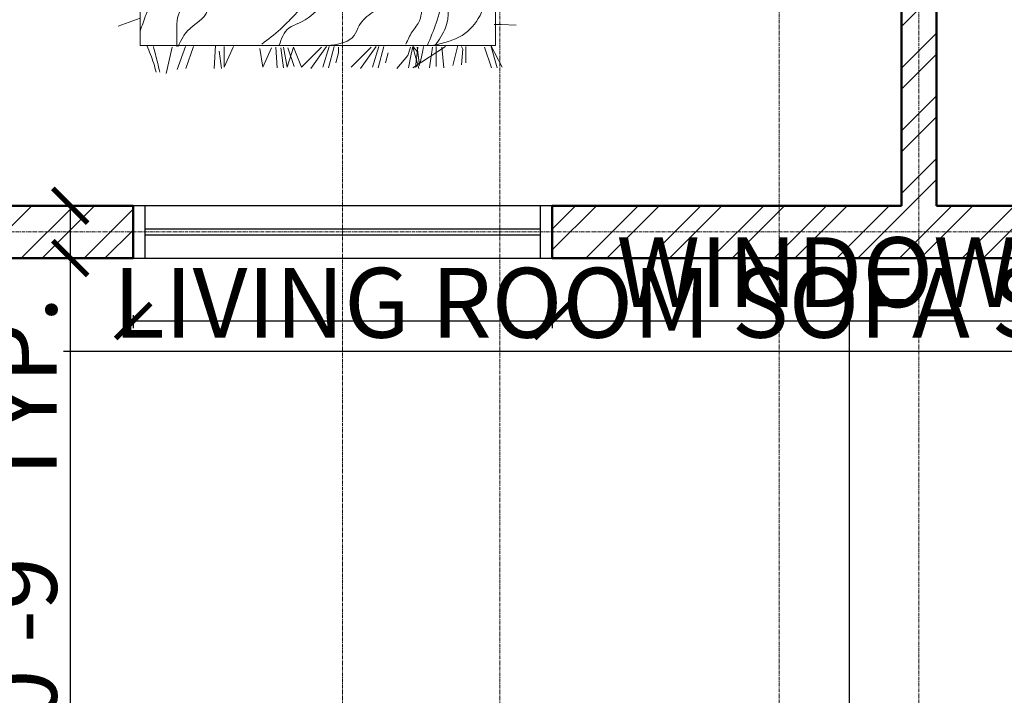
# Model space of a CAD drawing. Units: inches. Extents: x 261 to 2725, y 291 to 1454.
# Tile 4 of 35: x 519 to 688, y 433 to 549. Entities that reach past the tile are written whole.
import ezdxf

# ---------------------------------------------------------------- set-up
doc = ezdxf.new("R2010")
doc.units = ezdxf.units.IN
doc.linetypes.add('CENTER', pattern=[2, 1.25, -0.25, 0.25, -0.25])
for name, color, linetype, lineweight in [('A-ANNO-DIMS', 136, 'Continuous', 18), ('A-FLOR-STRS', 42, 'Continuous', 25), ('A-FURN', 30, 'Continuous', 18), ('A-GLAZ', 150, 'Continuous', 25), ('A-GRID', 251, 'CENTER', 13), ('A-WALL', 222, 'Continuous', 50), ('A-WALL-PATT', 243, 'Continuous', 13)]:
    doc.layers.add(name, color=color, linetype=linetype, lineweight=lineweight)
doc.styles.get("Standard").update_dxf_attribs({"font": 'arial.ttf'})
doc.dimstyles.new('ISO-25', dxfattribs={"dimtxt": 12, "dimasz": 6, "dimexe": 1.25, "dimexo": 0.625, "dimtad": 1, "dimdec": 0, "dimlunit": 3, "dimtxsty": 'Standard', "dimblk": 'ARCHTICK', "dimcen": 2.5, "dimadec": 0, "dimazin": 0, "dimtfac": 1, "dimtdec": 0, "dimtmove": 0, "dimatfit": 3, "dimfxl": 1, "dimfxlon": 1, "dimarcsym": 0})

# ---------------------------------------------------------------- blocks, each defined once
blk = doc.blocks.new('A$C2B723114')
for p, q in [((0.5047, 1.5819), (0.5353, 1.4945)), ((0.4269, 0.0884), (0.4269, 1.4945)), ((0.4269, 1.4945), (0.6794, 1.4945)), ((0.3172, 1.3923), (0.4213, 1.3687)), ((0.3318, 1.3485), (0.4241, 1.3149)), ((0.3367, 1.3143), (0.4241, 1.2838)), ((0.3367, 1.2016), (0.427, 1.1959)), ((0.3367, 1.1724), (0.405, 1.1821)), ((0.4241, 1.162), (0.3421, 1.162)), ((0.3421, 1.162), (0.4241, 1.1252)), ((0.4157, 1.0206), (0.3421, 1.0093)), ((0.3421, 1.0093), (0.4185, 0.9754)), ((0.4213, 0.9584), (0.3392, 0.9527)), ((0.4185, 0.9386), (0.3392, 0.9272)), ((0.4213, 0.9272), (0.3421, 0.9131)), ((0.3421, 0.9131), (0.4213, 0.8876)), ((0.4185, 0.9103), (0.3449, 0.8848)), ((0.4213, 0.8876), (0.3421, 0.8565)), ((0.3364, 0.8197), (0.4241, 0.7574)), ((0.3421, 0.8565), (0.4213, 0.7772)), ((0.3392, 0.7489), (0.4241, 0.7263)), ((0.3421, 0.7716), (0.4241, 0.7461)), ((0.359, 0.7206), (0.3987, 0.7093)), ((0.3987, 0.7093), (0.4213, 0.7093)), ((0.3421, 0.6601), (0.4213, 0.5808)), ((0.3364, 0.6233), (0.4241, 0.561)), ((0.3392, 0.5525), (0.4241, 0.5299)), ((0.3421, 0.5752), (0.4241, 0.5497)), ((0.359, 0.5242), (0.3987, 0.5129)), ((0.3364, 0.4785), (0.3874, 0.436)), ((0.3392, 0.4332), (0.393, 0.4219)), ((0.3874, 0.436), (0.4213, 0.4247)), ((0.4213, 0.415), (0.3364, 0.3923)), ((0.4241, 0.2868), (0.3392, 0.415)), ((0.3421, 0.4049), (0.3647, 0.3851)), ((0.4213, 0.3964), (0.3421, 0.4049)), ((0.4213, 0.398), (0.3477, 0.3895)), ((0.393, 0.4219), (0.4241, 0.4162)), ((0.4241, 0.4162), (0.4015, 0.3964)), ((0.3647, 0.3851), (0.4072, 0.3766)), ((0.4072, 0.3766), (0.4241, 0.3738)), ((0.4213, 0.3377), (0.3392, 0.3491)), ((0.4241, 0.3236), (0.3449, 0.3236)), ((0.3392, 0.2925), (0.4213, 0.3009)), ((0.3477, 0.2571), (0.427, 0.2373)), ((0.3506, 0.2231), (0.4128, 0.2175)), ((0.359, 0.2061), (0.4241, 0.2061)), ((0.4128, 0.2175), (0.4241, 0.2231)), ((0.3392, 0.1042), (0.4213, 0.1325)), ((0.3392, 0.0815), (0.427, 0.107)), ((0.427, 0.107), (0.3421, 0.0617)), ((2.4685, 0.0903), (0.4269, 0.0884)), ((0.5106, 0.094), (0.5106, 0.0657)), ((0.5106, 0.0657), (0.5077, 0.0063))]:
    blk.add_line(p, q)
for points, knots in [([(0.6768, 1.3104), (0.6615, 1.3339), (0.6315, 1.3797), (0.604, 1.4501), (0.5417, 1.4748), (0.5064, 1.4871), (0.4848, 1.4945)], [0, 0, 0, 0, 110.980521, 216.571322, 273.316778, 363.252298, 363.252298, 363.252298, 363.252298]), ([(0.427, 1.4678), (0.4036, 1.4582), (0.3693, 1.4441), (0.3335, 1.4344), (0.3221, 1.4313)], [0, 0, 0, 0, 98.452083, 144.639601, 144.639601, 144.639601, 144.639601]), ([(0.4241, 1.4423), (0.4031, 1.437), (0.3691, 1.4284), (0.3351, 1.4199), (0.3221, 1.4167)], [0, 0, 0, 0, 84.638756, 136.955563, 136.955563, 136.955563, 136.955563]), ([(0.6768, 1.286), (0.6567, 1.2911), (0.6145, 1.3017), (0.5543, 1.3533), (0.4816, 1.349), (0.4362, 1.3493), (0.4233, 1.3493)], [0, 0, 0, 0, 80.250278, 168.388677, 295.908361, 346.663112, 346.663112, 346.663112, 346.663112]), ([(0.4233, 1.3445), (0.4367, 1.3385), (0.464, 1.3264), (0.5129, 1.2848), (0.5456, 1.2161), (0.6131, 1.2349), (0.6142, 1.1913), (0.6642, 1.1806), (0.674, 1.144), (0.6817, 1.1154)], [0, 0, 0, 0, 56.745495, 115.23739, 254.956954, 286.678662, 337.828324, 366.201072, 468.500395, 468.500395, 468.500395, 468.500395]), ([(0.6817, 0.8034), (0.6673, 0.8119), (0.6341, 0.8315), (0.5785, 0.8518), (0.5349, 0.8973), (0.4828, 0.9461), (0.4518, 0.9879), (0.4331, 1.013)], [0, 0, 0, 0, 65.318952, 150.437229, 226.833166, 307.58338, 429.454095, 429.454095, 429.454095, 429.454095]), ([(0.4282, 0.9448), (0.4547, 0.9353), (0.496, 0.9206), (0.5223, 0.8436), (0.5628, 0.7946), (0.6113, 0.7575), (0.6214, 0.7173), (0.6539, 0.7022), (0.672, 0.6897), (0.6768, 0.6864)], [0, 0, 0, 0, 102.299436, 159.044876, 303.717955, 348.579152, 391.138254, 454.581655, 477.456496, 477.456496, 477.456496, 477.456496]), ([(0.4282, 0.74), (0.4347, 0.7029), (0.444, 0.6496), (0.5194, 0.6274), (0.555, 0.5807), (0.5975, 0.5243), (0.6789, 0.5415), (0.677, 0.5095), (0.6768, 0.5061)], [0, 0, 0, 0, 130.791737, 187.537266, 286.231946, 353.673191, 460.023761, 472.712403, 472.712403, 472.712403, 472.712403]), ([(0.4331, 0.4427), (0.4498, 0.4356), (0.4827, 0.4216), (0.5314, 0.3759), (0.632, 0.3884), (0.6996, 0.3513), (0.7423, 0.3278)], [0, 0, 0, 0, 70.931849, 139.556414, 248.154027, 434.709995, 434.709995, 434.709995, 434.709995]), ([(2.4625, 0.1088), (2.4095, 0.1438), (2.2904, 0.2226), (2.0623, 0.1771), (1.9006, 0.2246), (1.7699, 0.2337), (1.6941, 0.2766), (1.5528, 0.2786), (1.4005, 0.2587), (1.2324, 0.3267), (1.059, 0.2939), (0.9218, 0.426), (0.7359, 0.3204), (0.5586, 0.2391), (0.4502, 0.3116), (0.427, 0.3272)], [0, 0, 0, 0, 239.874704, 538.942419, 850.40885, 893.390315, 1047.998294, 1176.505142, 1437.500972, 1637.333004, 1864.324391, 2089.058767, 2248.736533, 2637.953392, 2744.252142, 2744.252142, 2744.252142, 2744.252142]), ([(1.9771, 0.0962), (1.9286, 0.1117), (1.7864, 0.157), (1.5223, 0.1992), (1.2611, 0.141), (1.0527, 0.2023), (0.8859, 0.1885), (0.76, 0.3042), (0.6211, 0.292), (0.5187, 0.3203), (0.4572, 0.3456), (0.4282, 0.3575)], [0, 0, 0, 0, 198.710624, 582.73994, 1031.873213, 1206.082894, 1423.278209, 1655.952104, 1808.744089, 1945.69963, 2068.229211, 2068.229211, 2068.229211, 2068.229211]), ([(0.8474, 0.0943), (0.82, 0.1047), (0.757, 0.1287), (0.6201, 0.1029), (0.4623, 0.1837), (0.4372, 0.2936), (0.4282, 0.3331)], [0, 0, 0, 0, 112.422038, 258.341957, 533.791494, 688.286079, 688.286079, 688.286079, 688.286079])]:
    blk.add_open_spline(points, degree=3, knots=knots)
blk = doc.blocks.new('_ArchTick')
at = {"color": 0, "linetype": 'ByBlock', "const_width": 0.15}
blk.add_lwpolyline([(-0.5, -0.5), (0.5, 0.5)], dxfattribs=at)
blk = doc.blocks.new('*D28')
at = {"layer": 'A-ANNO-DIMS', "color": 0, "lineweight": -2, "transparency": 16777216}
for p, q in [((469.45, 349.55), (469.45, 347.3)), ((469.45, 348.55), (955.45, 348.55)), ((955.45, 349.55), (955.45, 347.3))]:
    blk.add_line(p, q, dxfattribs=at)
at = {"layer": 'Defpoints', "color": 0, "transparency": 16777216}
for p in [(469.45, 508.47), (955.45, 508.47), (955.45, 348.55)]:
    blk.add_point(p, dxfattribs=at)
at = {"layer": 'A-ANNO-DIMS', "color": 0, "lineweight": -2, "transparency": 16777216, "xscale": 6, "yscale": 6, "zscale": 6, "rotation": 180}
blk.add_blockref('_ArchTick', (469.45, 348.55), dxfattribs=at)
at = {"layer": 'A-ANNO-DIMS', "color": 0, "lineweight": -2, "transparency": 16777216, "xscale": 6, "yscale": 6, "zscale": 6}
blk.add_blockref('_ArchTick', (955.45, 348.55), dxfattribs=at)
at = {"layer": 'A-ANNO-DIMS', "color": 0, "transparency": 16777216, "insert": (712.45, 355.3), "char_height": 12, "attachment_point": 5}
blk.add_mtext('40\'-6"', dxfattribs=at)
blk = doc.blocks.new('*D31')
at = {"layer": 'A-ANNO-DIMS', "color": 0, "lineweight": -2, "transparency": 16777216}
for p, q in [((478.45, 389.14), (478.45, 386.89)), ((946.45, 389.14), (946.45, 386.89)), ((478.45, 388.14), (946.45, 388.14))]:
    blk.add_line(p, q, dxfattribs=at)
at = {"layer": 'Defpoints', "color": 0, "transparency": 16777216}
for p in [(478.45, 517.47), (946.45, 517.47), (946.45, 388.14)]:
    blk.add_point(p, dxfattribs=at)
at = {"layer": 'A-ANNO-DIMS', "color": 0, "lineweight": -2, "transparency": 16777216, "xscale": 6, "yscale": 6, "zscale": 6, "rotation": 180}
blk.add_blockref('_ArchTick', (478.45, 388.14), dxfattribs=at)
at = {"layer": 'A-ANNO-DIMS', "color": 0, "lineweight": -2, "transparency": 16777216, "xscale": 6, "yscale": 6, "zscale": 6}
blk.add_blockref('_ArchTick', (946.45, 388.14), dxfattribs=at)
at = {"layer": 'A-ANNO-DIMS', "color": 0, "transparency": 16777216, "insert": (712.45, 394.89), "char_height": 12, "attachment_point": 5}
blk.add_mtext("39'", dxfattribs=at)
blk = doc.blocks.new('WIN-72')
for p, q in [((955.45, 950.47), (946.45, 950.47)), ((950.45, 950.47), (950.45, 882.47)), ((951.45, 882.47), (951.45, 950.47)), ((946.45, 882.47), (955.45, 882.47))]:
    blk.add_line(p, q)
blk.add_lwpolyline([(955.45, 880.47), (955.45, 952.47), (946.45, 952.47), (946.45, 880.47)], close=True)
blk = doc.blocks.new('*D39')
at = {"layer": 'A-ANNO-DIMS', "color": 0, "lineweight": -2, "ltscale": 0.07, "transparency": 16777216}
for p, q in [((538.45, 498.67), (538.45, 496.42)), ((538.45, 497.67), (610.45, 497.67)), ((610.45, 498.67), (610.45, 496.42)), ((610.45, 497.67), (799.35, 497.67))]:
    blk.add_line(p, q, dxfattribs=at)
at = {"layer": 'Defpoints', "color": 0, "ltscale": 0.07, "transparency": 16777216}
for p in [(538.45, 508.47), (610.45, 508.47), (610.45, 497.67)]:
    blk.add_point(p, dxfattribs=at)
at = {"layer": 'A-ANNO-DIMS', "color": 0, "lineweight": -2, "ltscale": 0.07, "transparency": 16777216, "xscale": 6, "yscale": 6, "zscale": 6, "rotation": 180}
blk.add_blockref('_ArchTick', (538.45, 497.67), dxfattribs=at)
at = {"layer": 'A-ANNO-DIMS', "color": 0, "lineweight": -2, "ltscale": 0.07, "transparency": 16777216, "xscale": 6, "yscale": 6, "zscale": 6}
blk.add_blockref('_ArchTick', (610.45, 497.67), dxfattribs=at)
at = {"layer": 'A-ANNO-DIMS', "color": 0, "ltscale": 0.07, "transparency": 16777216, "insert": (707.9, 504.5), "char_height": 12, "attachment_point": 5}
blk.add_mtext('WINDOW W1 6\'-0" TYP.', dxfattribs=at)
blk = doc.blocks.new('*D40')
at = {"layer": 'A-ANNO-DIMS', "color": 0, "lineweight": -2, "ltscale": 0.07, "transparency": 16777216}
for p, q in [((528.65, 517.47), (526.4, 517.47)), ((527.65, 517.47), (527.65, 508.47)), ((528.65, 508.47), (526.4, 508.47)), ((527.65, 508.47), (527.65, 428.07))]:
    blk.add_line(p, q, dxfattribs=at)
at = {"layer": 'Defpoints', "color": 0, "ltscale": 0.07, "transparency": 16777216}
for p in [(538.45, 517.47), (527.65, 508.47), (538.45, 508.47)]:
    blk.add_point(p, dxfattribs=at)
at = {"layer": 'A-ANNO-DIMS', "color": 0, "lineweight": -2, "ltscale": 0.07, "transparency": 16777216, "xscale": 6, "yscale": 6, "zscale": 6}
for p, rotation in [((527.65, 517.47), 90), ((527.65, 508.47), 270)]:
    blk.add_blockref('_ArchTick', p, dxfattribs=dict(at, rotation=rotation))
at = {"layer": 'A-ANNO-DIMS', "color": 0, "ltscale": 0.07, "transparency": 16777216, "insert": (520.9, 465.27), "char_height": 12, "attachment_point": 5, "rotation": 90}
blk.add_mtext('0\'-9" TYP.', dxfattribs=at)
blk = doc.blocks.new('*D67')
at = {"layer": 'A-ANNO-DIMS', "color": 0, "lineweight": -2, "ltscale": 0.07, "transparency": 16777216}
for p, q in [((778.45, 492.4), (526.52, 492.4)), ((778.45, 493.4), (778.45, 491.15)), ((946.45, 492.4), (778.45, 492.4)), ((946.45, 493.4), (946.45, 491.15))]:
    blk.add_line(p, q, dxfattribs=at)
at = {"layer": 'Defpoints', "color": 0, "ltscale": 0.07, "transparency": 16777216}
for p in [(778.45, 517.6), (946.45, 517.6), (778.45, 492.4)]:
    blk.add_point(p, dxfattribs=at)
at = {"layer": 'A-ANNO-DIMS', "color": 0, "lineweight": -2, "ltscale": 0.07, "transparency": 16777216, "xscale": 6, "yscale": 6, "zscale": 6, "rotation": 180}
blk.add_blockref('_ArchTick', (778.45, 492.4), dxfattribs=at)
at = {"layer": 'A-ANNO-DIMS', "color": 0, "lineweight": -2, "ltscale": 0.07, "transparency": 16777216, "xscale": 6, "yscale": 6, "zscale": 6}
blk.add_blockref('_ArchTick', (946.45, 492.4), dxfattribs=at)
at = {"layer": 'A-ANNO-DIMS', "color": 0, "ltscale": 0.07, "transparency": 16777216, "insert": (649.49, 499.24), "char_height": 12, "attachment_point": 5}
blk.add_mtext('LIVING ROOM SOFA SET 14\'-0"', dxfattribs=at)
blk = doc.blocks.new('*D86')
at = {"layer": 'A-ANNO-DIMS', "color": 0, "lineweight": -2, "ltscale": 0.07, "transparency": 16777216}
for p, q in [((676.45, 1437.76), (676.45, 1440.01)), ((772.45, 1437.76), (772.45, 1440.01)), ((676.45, 1438.76), (772.45, 1438.76))]:
    blk.add_line(p, q, dxfattribs=at)
at = {"layer": 'Defpoints', "color": 0, "ltscale": 0.07, "transparency": 16777216}
for p in [(772.45, 1438.76), (676.45, 517.47), (772.45, 517.47)]:
    blk.add_point(p, dxfattribs=at)
at = {"layer": 'A-ANNO-DIMS', "color": 0, "lineweight": -2, "ltscale": 0.07, "transparency": 16777216, "xscale": 6, "yscale": 6, "zscale": 6, "rotation": 180}
blk.add_blockref('_ArchTick', (676.45, 1438.76), dxfattribs=at)
at = {"layer": 'A-ANNO-DIMS', "color": 0, "lineweight": -2, "ltscale": 0.07, "transparency": 16777216, "xscale": 6, "yscale": 6, "zscale": 6}
blk.add_blockref('_ArchTick', (772.45, 1438.76), dxfattribs=at)
at = {"layer": 'A-ANNO-DIMS', "color": 0, "ltscale": 0.07, "transparency": 16777216, "insert": (724.45, 1445.51), "char_height": 12, "attachment_point": 5}
blk.add_mtext('8\'-0"', dxfattribs=at)
blk = doc.blocks.new('*D96')
at = {"layer": 'A-ANNO-DIMS', "color": 0, "lineweight": -2, "ltscale": 0.07, "transparency": 16777216}
for p, q in [((577.45, 305.22), (577.45, 302.97)), ((670.45, 305.22), (670.45, 302.97)), ((577.45, 304.22), (670.45, 304.22))]:
    blk.add_line(p, q, dxfattribs=at)
at = {"layer": 'Defpoints', "color": 0, "ltscale": 0.07, "transparency": 16777216}
for p in [(577.45, 775.47), (670.45, 775.47), (670.45, 304.22)]:
    blk.add_point(p, dxfattribs=at)
at = {"layer": 'A-ANNO-DIMS', "color": 0, "lineweight": -2, "ltscale": 0.07, "transparency": 16777216, "xscale": 6, "yscale": 6, "zscale": 6, "rotation": 180}
blk.add_blockref('_ArchTick', (577.45, 304.22), dxfattribs=at)
at = {"layer": 'A-ANNO-DIMS', "color": 0, "lineweight": -2, "ltscale": 0.07, "transparency": 16777216, "xscale": 6, "yscale": 6, "zscale": 6}
blk.add_blockref('_ArchTick', (670.45, 304.22), dxfattribs=at)
at = {"layer": 'A-ANNO-DIMS', "color": 0, "ltscale": 0.07, "transparency": 16777216, "insert": (623.95, 310.97), "char_height": 12, "attachment_point": 5}
blk.add_mtext('7\'-9"', dxfattribs=at)
blk = doc.blocks.new('*D103')
at = {"layer": 'A-ANNO-DIMS', "color": 0, "lineweight": -2, "ltscale": 0.07, "transparency": 16777216}
for p, q in [((287.06, 1231.47), (284.81, 1231.47)), ((286.06, 439.47), (286.06, 1231.47)), ((287.06, 439.47), (284.81, 439.47))]:
    blk.add_line(p, q, dxfattribs=at)
at = {"layer": 'Defpoints', "color": 0, "ltscale": 0.07, "transparency": 16777216}
for p in [(286.06, 1231.47), (1243.08, 1231.47), (1243.08, 439.47)]:
    blk.add_point(p, dxfattribs=at)
at = {"layer": 'A-ANNO-DIMS', "color": 0, "lineweight": -2, "ltscale": 0.07, "transparency": 16777216, "xscale": 6, "yscale": 6, "zscale": 6}
for p, rotation in [((286.06, 1231.47), 90), ((286.06, 439.47), 270)]:
    blk.add_blockref('_ArchTick', p, dxfattribs=dict(at, rotation=rotation))
at = {"layer": 'A-ANNO-DIMS', "color": 0, "ltscale": 0.07, "transparency": 16777216, "insert": (279.3, 835.47), "char_height": 12, "attachment_point": 5, "rotation": 90}
blk.add_mtext('66\'-0"', dxfattribs=at)
blk = doc.blocks.new('*D106')
at = {"layer": 'A-ANNO-DIMS', "color": 0, "lineweight": -2, "ltscale": 0.07, "transparency": 16777216}
for p, q in [((287.06, 496.47), (284.81, 496.47)), ((286.06, 448.47), (286.06, 496.47)), ((287.06, 448.47), (284.81, 448.47))]:
    blk.add_line(p, q, dxfattribs=at)
at = {"layer": 'Defpoints', "color": 0, "ltscale": 0.07, "transparency": 16777216}
for p in [(286.06, 496.47), (1252.08, 496.47), (1252.08, 448.47)]:
    blk.add_point(p, dxfattribs=at)
at = {"layer": 'A-ANNO-DIMS', "color": 0, "lineweight": -2, "ltscale": 0.07, "transparency": 16777216, "xscale": 6, "yscale": 6, "zscale": 6}
for p, rotation in [((286.06, 496.47), 90), ((286.06, 448.47), 270)]:
    blk.add_blockref('_ArchTick', p, dxfattribs=dict(at, rotation=rotation))
at = {"layer": 'A-ANNO-DIMS', "color": 0, "ltscale": 0.07, "transparency": 16777216, "insert": (279.3, 472.47), "char_height": 12, "attachment_point": 5, "rotation": 90}
blk.add_mtext('4\'-0"', dxfattribs=at)
blk = doc.blocks.new('*D107')
at = {"layer": 'A-ANNO-DIMS', "color": 0, "lineweight": -2, "ltscale": 0.07, "transparency": 16777216}
for p, q in [((287.06, 673.47), (284.81, 673.47)), ((286.06, 496.47), (286.06, 673.47)), ((287.06, 496.47), (284.81, 496.47))]:
    blk.add_line(p, q, dxfattribs=at)
at = {"layer": 'Defpoints', "color": 0, "ltscale": 0.07, "transparency": 16777216}
for p in [(286.06, 673.47), (1252.08, 673.47), (1252.08, 496.47)]:
    blk.add_point(p, dxfattribs=at)
at = {"layer": 'A-ANNO-DIMS', "color": 0, "lineweight": -2, "ltscale": 0.07, "transparency": 16777216, "xscale": 6, "yscale": 6, "zscale": 6}
for p, rotation in [((286.06, 673.47), 90), ((286.06, 496.47), 270)]:
    blk.add_blockref('_ArchTick', p, dxfattribs=dict(at, rotation=rotation))
at = {"layer": 'A-ANNO-DIMS', "color": 0, "ltscale": 0.07, "transparency": 16777216, "insert": (279.3, 584.97), "char_height": 12, "attachment_point": 5, "rotation": 90}
blk.add_mtext('14\'-9"', dxfattribs=at)
blk = doc.blocks.new('*D123')
at = {"layer": 'A-ANNO-DIMS', "color": 0, "lineweight": -2, "ltscale": 0.07, "transparency": 16777216}
for p, q in [((287.06, 1054.85), (284.81, 1054.85)), ((286.06, 439.47), (286.06, 1054.85)), ((287.06, 439.47), (284.81, 439.47))]:
    blk.add_line(p, q, dxfattribs=at)
at = {"layer": 'Defpoints', "color": 0, "ltscale": 0.07, "transparency": 16777216}
for p in [(286.06, 1054.85), (2007.71, 1054.85), (2007.71, 439.47)]:
    blk.add_point(p, dxfattribs=at)
at = {"layer": 'A-ANNO-DIMS', "color": 0, "lineweight": -2, "ltscale": 0.07, "transparency": 16777216, "xscale": 6, "yscale": 6, "zscale": 6}
for p, rotation in [((286.06, 1054.85), 90), ((286.06, 439.47), 270)]:
    blk.add_blockref('_ArchTick', p, dxfattribs=dict(at, rotation=rotation))
at = {"layer": 'A-ANNO-DIMS', "color": 0, "ltscale": 0.07, "transparency": 16777216, "insert": (279.22, 747.16), "char_height": 12, "attachment_point": 5, "rotation": 90}
blk.add_mtext('51\'-3 1/2"', dxfattribs=at)

msp = doc.modelspace()

# ---------------------------------------------------------------- hatches: boundary and pattern name
at = {"layer": 'A-WALL-PATT'}
h = msp.add_hatch(dxfattribs=at)
h.set_pattern_fill('ANSI32', color=256, scale=0.8)
h.paths.add_polyline_path([(478.45, 685.47), (580.45, 685.47), (580.45, 691.47), (577.45, 691.47), (577.45, 694.47), (571.45, 694.47), (571.45, 691.47), (478.45, 691.47), (478.45, 721.47), (469.45, 721.47), (469.45, 508.47), (538.45, 508.47), (538.45, 517.47), (478.45, 517.47)])
h.paths.add_polyline_path([(694.45, 517.47), (676.45, 517.47), (676.45, 646.47), (670.45, 646.47), (670.45, 517.47), (610.45, 517.47), (610.45, 508.47), (694.45, 508.47)])
h.paths.add_polyline_path([(676.45, 784.47), (478.45, 784.47), (478.45, 844.47), (469.45, 844.47), (469.45, 745.47), (478.45, 745.47), (478.45, 775.47), (571.45, 775.47), (571.45, 724.47), (577.45, 724.47), (577.45, 775.47), (670.45, 775.47), (670.45, 691.47), (610.45, 691.47), (610.45, 685.47), (670.45, 685.47), (670.45, 682.47), (676.45, 682.47)])
h.paths.add_polyline_path([(955.45, 880.47), (946.45, 880.47), (946.45, 808.47), (778.45, 808.47), (778.45, 799.47), (946.45, 799.47), (946.45, 517.47), (898.45, 517.47), (898.45, 508.47), (955.45, 508.47)])
h.paths.add_polyline_path([(778.45, 598.47), (772.45, 598.47), (772.45, 517.47), (754.45, 517.47), (754.45, 508.47), (826.45, 508.47), (826.45, 517.47), (778.45, 517.47)])
h.paths.add_polyline_path([(955.45, 1090.47), (946.45, 1090.47), (946.45, 1030.47), (817.45, 1030.47), (817.45, 1024.47), (946.45, 1024.47), (946.45, 952.47), (955.45, 952.47)])
h.paths.add_polyline_path([(955.45, 1231.47), (730.45, 1231.47), (730.45, 1222.47), (772.45, 1222.47), (772.45, 1096.47), (766.45, 1096.47), (766.45, 1090.47), (772.45, 1090.47), (772.45, 1006.47), (712.45, 1006.47), (712.45, 1000.47), (778.45, 1000.47), (778.45, 1024.47), (781.45, 1024.47), (781.45, 1030.47), (778.45, 1030.47), (778.45, 1222.47), (946.45, 1222.47), (946.45, 1162.47), (955.45, 1162.47)])
h.paths.add_polyline_path([(694.45, 1231.47), (619.45, 1231.47), (619.45, 1222.47), (646.45, 1222.47), (646.45, 1039.47), (652.45, 1039.47), (652.45, 1090.47), (736.45, 1090.47), (736.45, 1096.47), (652.45, 1096.47), (652.45, 1222.47), (694.45, 1222.47)])
h.paths.add_polyline_path([(571.45, 1231.47), (469.45, 1231.47), (469.45, 1099.47), (478.45, 1099.47), (478.45, 1144.47), (544.45, 1144.47), (544.45, 1153.47), (538.45, 1153.47), (538.45, 1150.47), (478.45, 1150.47), (478.45, 1222.47), (538.45, 1222.47), (538.45, 1183.47), (544.45, 1183.47), (544.45, 1222.47), (571.45, 1222.47)])
h.paths.add_polyline_path([(538.45, 1006.47), (478.45, 1006.47), (478.45, 1051.47), (469.45, 1051.47), (469.45, 940.47), (478.45, 940.47), (478.45, 1000.47), (538.45, 1000.47)])
h.paths.add_polyline_path([(652.45, 1006.47), (652.45, 1009.47), (646.45, 1009.47), (646.45, 1006.47), (586.45, 1006.47), (586.45, 1000.47), (652.45, 1000.47)])
h.paths.add_polyline_path([(1288.08, 973.47), (1243.08, 973.47), (1243.08, 920.97), (1252.08, 920.97), (1252.08, 964.47), (1288.08, 964.47)], flags=17)
h.paths.add_polyline_path([(1402.08, 805.47), (1252.08, 805.47), (1252.08, 848.97), (1243.08, 848.97), (1243.08, 757.47), (1252.08, 757.47), (1252.08, 799.47), (1294.08, 799.47), (1372.08, 799.47), (1372.08, 779.47), (1372.08, 715.47), (1378.08, 715.47), (1378.08, 799.47), (1402.08, 799.47)])
h.paths.add_polyline_path([(1252.08, 721.47), (1243.08, 721.47), (1243.08, 439.47), (1729.08, 439.47), (1729.08, 709.47), (1720.08, 709.47), (1720.08, 679.47), (1582.08, 679.47), (1582.08, 670.47), (1588.08, 670.47), (1588.08, 673.47), (1720.08, 673.47), (1720.08, 559.47), (1690.08, 559.47), (1690.08, 550.47), (1720.08, 550.47), (1720.08, 448.47), (1252.08, 448.47), (1252.08, 496.47), (1312.08, 496.47), (1312.08, 505.47), (1252.08, 505.47), (1252.08, 673.47), (1405.08, 673.47), (1405.08, 679.47), (1378.08, 679.47), (1378.08, 685.47), (1372.08, 685.47), (1372.08, 679.47), (1252.08, 679.47)])
h.paths.add_polyline_path([(1450.08, 550.47), (1480.08, 550.47), (1480.08, 559.47), (1450.08, 559.47), (1450.08, 679.47), (1441.08, 679.47), (1441.08, 673.47), (1444.08, 673.47), (1444.08, 505.47), (1384.08, 505.47), (1384.08, 496.47), (1450.08, 496.47)], flags=17)
h.paths.add_polyline_path([(1618.08, 559.47), (1588.08, 559.47), (1588.08, 634.47), (1582.08, 634.47), (1582.08, 559.47), (1552.08, 559.47), (1552.08, 550.47), (1618.08, 550.47)], flags=17)
h.paths.add_polyline_path([(1564.08, 964.47), (1630.08, 964.47), (1630.08, 973.47), (1477.08, 973.47), (1477.08, 964.47), (1558.08, 964.47), (1558.08, 926.22), (1558.08, 887.97), (1486.08, 887.97), (1486.08, 881.97), (1558.08, 881.97), (1558.08, 805.47), (1450.08, 805.47), (1450.08, 845.97), (1444.08, 845.97), (1444.08, 805.47), (1438.08, 805.47), (1438.08, 799.47), (1564.08, 799.47)], flags=17)
h.paths.add_polyline_path([(1453.08, 973.47), (1408.08, 973.47), (1408.08, 964.47), (1444.08, 964.47), (1444.08, 881.97), (1450.08, 881.97), (1456.08, 881.97), (1456.08, 887.97), (1450.08, 887.97), (1450.08, 964.47), (1453.08, 964.47)], flags=17)
h.paths.add_polyline_path([(1729.08, 1231.47), (1243.08, 1231.47), (1243.08, 1167.47), (1252.08, 1167.47), (1252.08, 1222.47), (1441.08, 1222.47), (1441.08, 1045.47), (1648.08, 1045.47), (1648.08, 1051.47), (1450.08, 1051.47), (1450.08, 1074.47), (1450.08, 1222.47), (1472.08, 1222.47), (1720.08, 1222.47), (1720.08, 1051.47), (1708.08, 1051.47), (1708.08, 1045.47), (1720.08, 1045.47), (1720.08, 973.47), (1702.08, 973.47), (1702.08, 964.47), (1720.08, 964.47), (1720.08, 769.47), (1729.08, 769.47)])
h.paths.add_polyline_path([(2493.71, 1054.85), (2007.71, 1054.85), (2007.71, 439.47), (2214.67, 439.47), (2214.67, 496.47), (2493.71, 496.47)])
h.paths.add_polyline_path([(2016.71, 1045.85), (2304.71, 1045.85), (2304.71, 841.47), (2310.71, 841.47), (2310.71, 1045.85), (2484.71, 1045.85), (2484.71, 805.47), (2310.71, 805.47), (2310.71, 811.47), (2304.71, 811.47), (2304.71, 799.47), (2484.71, 799.47), (2484.71, 679.47), (2304.71, 679.47), (2304.71, 673.47), (2484.71, 673.47), (2484.71, 505.47), (2208.67, 505.47), (2208.67, 448.47), (2016.71, 448.47), (2016.71, 799.47), (2304.71, 799.47), (2304.71, 805.47), (2016.71, 805.47)], flags=16)

# ---------------------------------------------------------------- linework, layer by layer
at = {"layer": 'A-FLOR-STRS'}
msp.add_line((661.45, 508.47), (661.45, 412.47), dxfattribs=at)
at = {"layer": 'A-GRID', "ltscale": 0.5}
for p, q in [((574.45, 1330.18), (574.45, 416.18)), ((601.45, 1330.18), (601.45, 416.18)), ((649.45, 1330.51), (649.45, 416.51)), ((673.45, 1330.51), (673.45, 416.51)), ((394.31, 512.97), (1018.31, 512.97))]:
    msp.add_line(p, q, dxfattribs=at)
at = {"layer": 'A-WALL'}
for p, q in [((670.45, 517.47), (670.45, 646.47)), ((676.45, 517.47), (676.45, 646.47)), ((478.45, 517.47), (538.45, 517.47)), ((538.45, 517.47), (538.45, 508.47)), ((610.45, 517.47), (610.45, 508.47)), ((610.45, 517.47), (670.45, 517.47)), ((676.45, 517.47), (694.45, 517.47)), ((469.45, 508.47), (538.45, 508.47)), ((610.45, 508.47), (694.45, 508.47))]:
    msp.add_line(p, q, dxfattribs=at)

# ---------------------------------------------------------------- block references
at = {"layer": 'A-FURN', "xscale": 43.4111919502411, "yscale": 43.4111919502411, "zscale": 43.4111919502411, "rotation": 90}
msp.add_blockref('A$C2B723114', (604.55, 526.47), dxfattribs=at)
at = {"layer": 'A-GLAZ', "rotation": 269.9999999999997}
msp.add_blockref('WIN-72', (-342.02, 1463.92), dxfattribs=at)

# ---------------------------------------------------------------- dimensions: what is measured, and where the dimension line sits
at = {"layer": 'A-ANNO-DIMS', "ltscale": 0.07}
for base, p1, p2, picture, middle in [((772.45, 1438.76), (676.45, 517.47), (772.45, 517.47), '*D86', (724.45, 1445.51)), ((670.45, 304.22), (577.45, 775.47), (670.45, 775.47), '*D96', (623.95, 310.97))]:
    dim = msp.add_linear_dim(base=base, p1=p1, p2=p2, dimstyle='ISO-25', override={"dimdec": 1, "dimlfac": 1, "dimrnd": 0, "dimzin": 1, "dimdsep": 46, "dimlunit": 4, "dimfrac": 2}, dxfattribs=at)
    dim.commit()
    dim.dimension.update_dxf_attribs({"geometry": picture, "text_midpoint": middle})
for base, p1, p2, picture, middle in [((286.06, 1231.47), (1243.08, 439.47), (1243.08, 1231.47), '*D103', (279.3, 835.47)), ((286.06, 1054.85), (2007.71, 439.47), (2007.71, 1054.85), '*D123', (279.22, 747.16)), ((286.06, 673.47), (1252.08, 496.47), (1252.08, 673.47), '*D107', (279.3, 584.97)), ((286.06, 496.47), (1252.08, 448.47), (1252.08, 496.47), '*D106', (279.3, 472.47))]:
    dim = msp.add_linear_dim(base=base, p1=p1, p2=p2, angle=90, dimstyle='ISO-25', override={"dimdec": 1, "dimlfac": 1, "dimrnd": 0, "dimzin": 1, "dimdsep": 46, "dimlunit": 4, "dimfrac": 2}, dxfattribs=at)
    dim.commit()
    dim.dimension.update_dxf_attribs({"geometry": picture, "text_midpoint": middle})
for base, p1, p2, angle, text, picture, middle in [((778.45, 492.4), (946.45, 517.6), (778.45, 517.6), 180, 'LIVING ROOM SOFA SET <>', '*D67', (649.49, 499.24)), ((527.65, 508.47), (538.45, 517.47), (538.45, 508.47), 270, '<> TYP.', '*D40', (520.9, 465.27))]:
    dim = msp.add_linear_dim(base=base, p1=p1, p2=p2, angle=angle, text=text, dimstyle='ISO-25', override={"dimdec": 1, "dimrnd": 0, "dimzin": 1, "dimlunit": 4, "dimfrac": 2}, dxfattribs=at)
    dim.commit()
    dim.dimension.update_dxf_attribs({"geometry": picture, "text_midpoint": middle})
dim = msp.add_linear_dim(base=(610.45, 497.67), p1=(538.45, 508.47), p2=(610.45, 508.47), text='WINDOW W1 <> TYP.', dimstyle='ISO-25', override={"dimdec": 1, "dimrnd": 0, "dimzin": 1, "dimlunit": 4, "dimfrac": 2}, dxfattribs=at)
dim.commit()
dim.dimension.update_dxf_attribs({"geometry": '*D39', "text_midpoint": (707.9, 504.5)})
at = {"layer": 'A-ANNO-DIMS'}
for base, p1, p2, picture, middle in [((946.45, 388.14), (478.45, 517.47), (946.45, 517.47), '*D31', (712.45, 388.14)), ((955.45, 348.55), (469.45, 508.47), (955.45, 508.47), '*D28', (712.45, 348.55))]:
    dim = msp.add_linear_dim(base=base, p1=p1, p2=p2, dimstyle='ISO-25', override={"dimclrd": 0, "dimclre": 0, "dimclrt": 0}, dxfattribs=at)
    dim.commit()
    dim.dimension.update_dxf_attribs({"geometry": picture, "text_midpoint": middle, "dimtype": 160})

doc.saveas('drawing.dxf')
